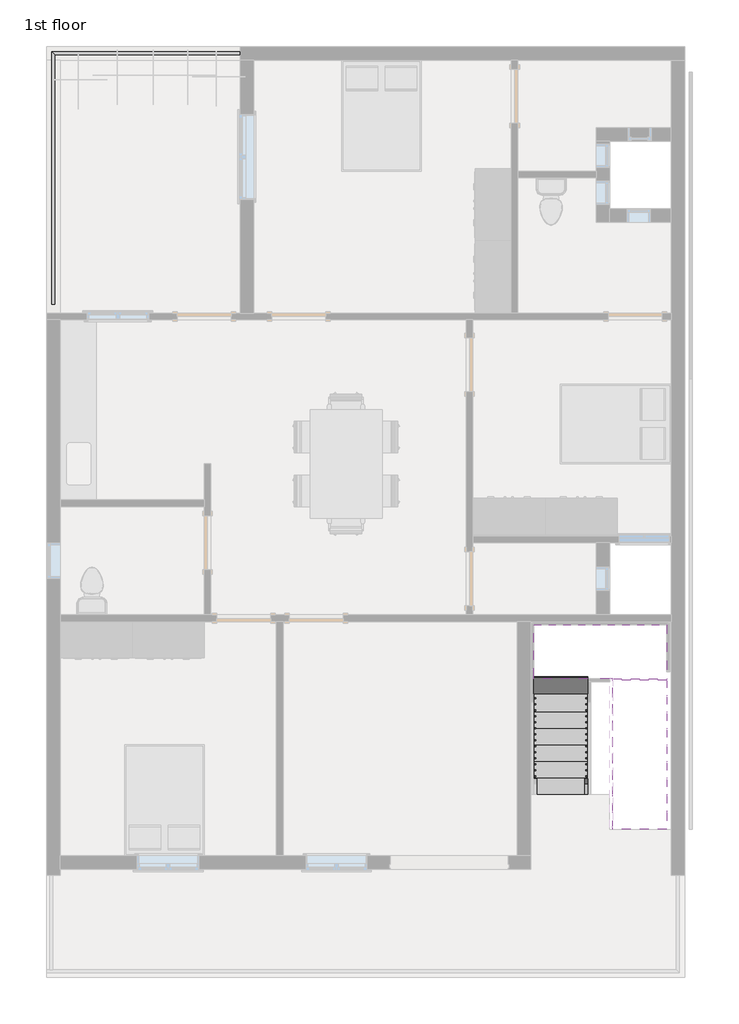
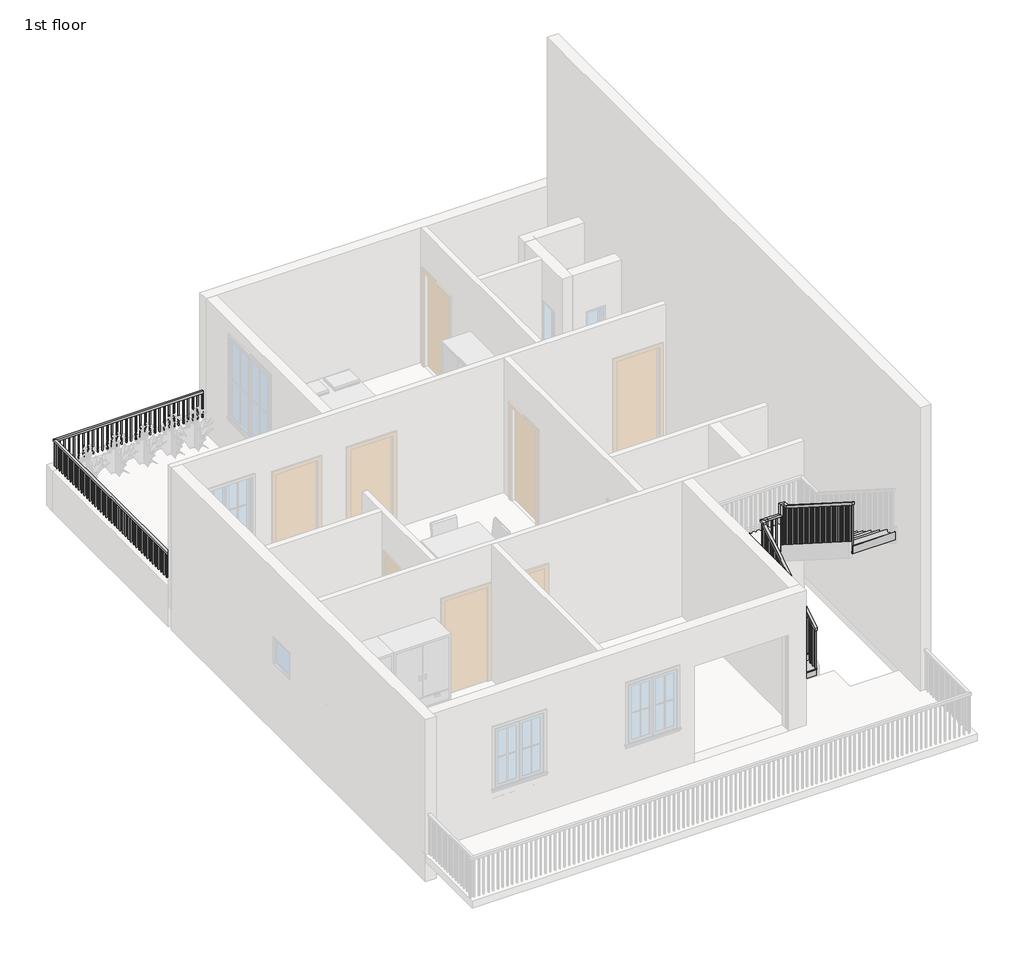
# One storey, part 3 of 5: 2 railings, 2 stair flights, 1 slab.
"""IFC4 building model written with IfcOpenShell, lengths in millimetres."""

from ifc_helpers import new_model, si_unit, frame, origin, place, context, project, spatial, polyline, outline, extrude, faceted_brep, transform, mapped, element, save
from components import non_monolithic_landing_85b13ac5, stair_flight_57d74f5f, stair_flight_b4f684d8

model = new_model("IFC4")

# Units and contexts
model_context = context("Model", 3, world=origin())
ifc_project = project(units=[si_unit("LENGTHUNIT", "METRE", prefix="MILLI")], contexts=[model_context])

# Site, building, storey
site = spatial("IfcSite", under=ifc_project)
building = spatial("IfcBuilding", under=site)
storey = spatial("IfcBuildingStorey", under=building, Name="1st floor", Elevation=3810.0)

# Railings
placement = place(None, origin())
element("IfcRailing", 1, ObjectType="Handrail - Rectangular", at=placement, inside=storey, context=model_context, shape_type="SolidModel", body=[
    faceted_brep([(995.5501403, 157.6257925, 4902.2), (995.5501403, 157.6257925, 4841.986276), (1046.3501403, 157.6257925, 4841.986276), (1046.3501403, 157.6257925, 4902.2), (995.5501403, 2037.2257925, 6098.3090909), (995.5501403, 2088.0257925, 6070.4226396), (1046.3501403, 2088.0257925, 6070.4226396), (1046.3501403, 2037.2257925, 6098.3090909), (995.5501403, 2037.2257925, 6146.8), (995.5501403, 2088.0257925, 6096.0), (1046.3501403, 2088.0257925, 6096.0), (1046.3501403, 2037.2257925, 6146.8), (995.5501403, 2164.2257925, 6146.8), (995.5501403, 2164.2257925, 6096.0), (1046.3501403, 2113.4257925, 6096.0), (1046.3501403, 2113.4257925, 6146.8), (1122.5501403, 2164.2257925, 6146.8), (1122.5501403, 2164.2257925, 6096.0), (1122.5501403, 2113.4257925, 6096.0), (1122.5501403, 2113.4257925, 6146.8), (1389.2501403, 2164.2257925, 6146.8), (1440.0501403, 2164.2257925, 6096.0), (1440.0501403, 2113.4257925, 6096.0), (1389.2501403, 2113.4257925, 6146.8), (1389.2501403, 2164.2257925, 6373.0909091), (1440.0501403, 2164.2257925, 6322.2909091), (1440.0501403, 2113.4257925, 6322.2909091), (1389.2501403, 2113.4257925, 6373.0909091), (1516.2501403, 2164.2257925, 6373.0909091), (1516.2501403, 2164.2257925, 6322.2909091), (1465.4501403, 2113.4257925, 6322.2909091), (1465.4501403, 2113.4257925, 6373.0909091), (1516.2501403, 2037.2257925, 6373.0909091), (1516.2501403, 2022.4327976, 6322.2909091), (1465.4501403, 2022.4327976, 6322.2909091), (1465.4501403, 2037.2257925, 6373.0909091), (1516.2501403, -401.1742075, 7924.8), (1465.4501403, -401.1742075, 7924.8), (1465.4501403, -401.1742075, 7864.586276), (1516.2501403, -401.1742075, 7864.586276)], [[[0, 1, 2, 3]], [[1, 0, 4, 5]], [[2, 1, 5, 6]], [[3, 2, 6, 7]], [[0, 3, 7, 4]], [[5, 4, 8, 9]], [[6, 5, 9, 10]], [[7, 6, 10, 11]], [[4, 7, 11, 8]], [[9, 8, 12, 13]], [[10, 9, 13, 14]], [[11, 10, 14, 15]], [[8, 11, 15, 12]], [[13, 12, 16, 17]], [[14, 13, 17, 18]], [[15, 14, 18, 19]], [[12, 15, 19, 16]], [[17, 16, 20, 21]], [[18, 17, 21, 22]], [[19, 18, 22, 23]], [[16, 19, 23, 20]], [[21, 20, 24, 25]], [[22, 21, 25, 26]], [[23, 22, 26, 27]], [[20, 23, 27, 24]], [[25, 24, 28, 29]], [[26, 25, 29, 30]], [[27, 26, 30, 31]], [[24, 27, 31, 28]], [[29, 28, 32, 33]], [[30, 29, 33, 34]], [[31, 30, 34, 35]], [[28, 31, 35, 32]], [[36, 37, 38, 39]], [[33, 32, 36, 39]], [[34, 33, 39, 38]], [[35, 34, 38, 37]], [[32, 35, 37, 36]]]),
    extrude(outline(polyline([(-309.0992075, 7805.9930941), (-290.0492075, 7793.8703669), (-290.0492075, 6832.6), (-309.0992075, 6832.6), (-309.0992075, 7805.9930941)])), frame((1481.3251403, 0.0, 0.0), z_axis=(1.0, 0.0, 0.0), x_axis=(0.0, 1.0, 0.0)), (0.0, 0.0, 1.0), 19.05),
    extrude(outline(polyline([(-207.4992075, 7741.3385487), (-188.4492075, 7729.2158214), (-188.4492075, 6832.6), (-207.4992075, 6832.6), (-207.4992075, 7741.3385487)])), frame((1481.3251403, 0.0, 0.0), z_axis=(1.0, 0.0, 0.0), x_axis=(0.0, 1.0, 0.0)), (0.0, 0.0, 1.0), 19.05),
    extrude(outline(polyline([(-105.8992075, 7676.6840032), (-86.8492075, 7664.561276), (-86.8492075, 6654.8), (-105.8992075, 6654.8), (-105.8992075, 7676.6840032)])), frame((1481.3251403, 0.0, 0.0), z_axis=(1.0, 0.0, 0.0), x_axis=(0.0, 1.0, 0.0)), (0.0, 0.0, 1.0), 19.05),
    extrude(outline(polyline([(-4.2992075, 7612.0294578), (14.7507925, 7599.9067305), (14.7507925, 6654.8), (-4.2992075, 6654.8), (-4.2992075, 7612.0294578)])), frame((1481.3251403, 0.0, 0.0), z_axis=(1.0, 0.0, 0.0), x_axis=(0.0, 1.0, 0.0)), (0.0, 0.0, 1.0), 19.05),
    extrude(outline(polyline([(97.3007925, 7547.3749123), (116.3507925, 7535.2521851), (116.3507925, 6654.8), (97.3007925, 6654.8), (97.3007925, 7547.3749123)])), frame((1481.3251403, 0.0, 0.0), z_axis=(1.0, 0.0, 0.0), x_axis=(0.0, 1.0, 0.0)), (0.0, 0.0, 1.0), 19.05),
    extrude(outline(polyline([(198.9007925, 7482.7203669), (217.9507925, 7470.5976396), (217.9507925, 6477.0), (198.9007925, 6477.0), (198.9007925, 7482.7203669)])), frame((1481.3251403, 0.0, 0.0), z_axis=(1.0, 0.0, 0.0), x_axis=(0.0, 1.0, 0.0)), (0.0, 0.0, 1.0), 19.05),
    extrude(outline(polyline([(300.5007925, 7418.0658214), (319.5507925, 7405.9430941), (319.5507925, 6477.0), (300.5007925, 6477.0), (300.5007925, 7418.0658214)])), frame((1481.3251403, 0.0, 0.0), z_axis=(1.0, 0.0, 0.0), x_axis=(0.0, 1.0, 0.0)), (0.0, 0.0, 1.0), 19.05),
    extrude(outline(polyline([(402.1007925, 7353.411276), (421.1507925, 7341.2885487), (421.1507925, 6477.0), (402.1007925, 6477.0), (402.1007925, 7353.411276)])), frame((1481.3251403, 0.0, 0.0), z_axis=(1.0, 0.0, 0.0), x_axis=(0.0, 1.0, 0.0)), (0.0, 0.0, 1.0), 19.05),
    extrude(outline(polyline([(503.7007925, 7288.7567305), (522.7507925, 7276.6340032), (522.7507925, 6299.2), (503.7007925, 6299.2), (503.7007925, 7288.7567305)])), frame((1481.3251403, 0.0, 0.0), z_axis=(1.0, 0.0, 0.0), x_axis=(0.0, 1.0, 0.0)), (0.0, 0.0, 1.0), 19.05),
    extrude(outline(polyline([(605.3007925, 7224.1021851), (624.3507925, 7211.9794578), (624.3507925, 6299.2), (605.3007925, 6299.2), (605.3007925, 7224.1021851)])), frame((1481.3251403, 0.0, 0.0), z_axis=(1.0, 0.0, 0.0), x_axis=(0.0, 1.0, 0.0)), (0.0, 0.0, 1.0), 19.05),
    extrude(outline(polyline([(706.9007925, 7159.4476396), (725.9507925, 7147.3249123), (725.9507925, 6299.2), (706.9007925, 6299.2), (706.9007925, 7159.4476396)])), frame((1481.3251403, 0.0, 0.0), z_axis=(1.0, 0.0, 0.0), x_axis=(0.0, 1.0, 0.0)), (0.0, 0.0, 1.0), 19.05),
    extrude(outline(polyline([(808.5007925, 7094.7930941), (827.5507925, 7082.6703669), (827.5507925, 6121.4), (808.5007925, 6121.4), (808.5007925, 7094.7930941)])), frame((1481.3251403, 0.0, 0.0), z_axis=(1.0, 0.0, 0.0), x_axis=(0.0, 1.0, 0.0)), (0.0, 0.0, 1.0), 19.05),
    extrude(outline(polyline([(910.1007925, 7030.1385487), (929.1507925, 7018.0158214), (929.1507925, 6121.4), (910.1007925, 6121.4), (910.1007925, 7030.1385487)])), frame((1481.3251403, 0.0, 0.0), z_axis=(1.0, 0.0, 0.0), x_axis=(0.0, 1.0, 0.0)), (0.0, 0.0, 1.0), 19.05),
    extrude(outline(polyline([(1011.7007925, 6965.4840032), (1030.7507925, 6953.361276), (1030.7507925, 5943.6), (1011.7007925, 5943.6), (1011.7007925, 6965.4840032)])), frame((1481.3251403, 0.0, 0.0), z_axis=(1.0, 0.0, 0.0), x_axis=(0.0, 1.0, 0.0)), (0.0, 0.0, 1.0), 19.05),
    extrude(outline(polyline([(1113.3007925, 6900.8294578), (1132.3507925, 6888.7067305), (1132.3507925, 5943.6), (1113.3007925, 5943.6), (1113.3007925, 6900.8294578)])), frame((1481.3251403, 0.0, 0.0), z_axis=(1.0, 0.0, 0.0), x_axis=(0.0, 1.0, 0.0)), (0.0, 0.0, 1.0), 19.05),
    extrude(outline(polyline([(1214.9007925, 6836.1749123), (1233.9507925, 6824.0521851), (1233.9507925, 5943.6), (1214.9007925, 5943.6), (1214.9007925, 6836.1749123)])), frame((1481.3251403, 0.0, 0.0), z_axis=(1.0, 0.0, 0.0), x_axis=(0.0, 1.0, 0.0)), (0.0, 0.0, 1.0), 19.05),
    extrude(outline(polyline([(1316.5007925, 6771.5203669), (1335.5507925, 6759.3976396), (1335.5507925, 5765.8), (1316.5007925, 5765.8), (1316.5007925, 6771.5203669)])), frame((1481.3251403, 0.0, 0.0), z_axis=(1.0, 0.0, 0.0), x_axis=(0.0, 1.0, 0.0)), (0.0, 0.0, 1.0), 19.05),
    extrude(outline(polyline([(1418.1007925, 6706.8658214), (1437.1507925, 6694.7430941), (1437.1507925, 5765.8), (1418.1007925, 5765.8), (1418.1007925, 6706.8658214)])), frame((1481.3251403, 0.0, 0.0), z_axis=(1.0, 0.0, 0.0), x_axis=(0.0, 1.0, 0.0)), (0.0, 0.0, 1.0), 19.05),
    extrude(outline(polyline([(1519.7007925, 6642.211276), (1538.7507925, 6630.0885487), (1538.7507925, 5765.8), (1519.7007925, 5765.8), (1519.7007925, 6642.211276)])), frame((1481.3251403, 0.0, 0.0), z_axis=(1.0, 0.0, 0.0), x_axis=(0.0, 1.0, 0.0)), (0.0, 0.0, 1.0), 19.05),
    extrude(outline(polyline([(1621.3007925, 6577.5567305), (1640.3507925, 6565.4340032), (1640.3507925, 5588.0), (1621.3007925, 5588.0), (1621.3007925, 6577.5567305)])), frame((1481.3251403, 0.0, 0.0), z_axis=(1.0, 0.0, 0.0), x_axis=(0.0, 1.0, 0.0)), (0.0, 0.0, 1.0), 19.05),
    extrude(outline(polyline([(1722.9007925, 6512.9021851), (1741.9507925, 6500.7794578), (1741.9507925, 5588.0), (1722.9007925, 5588.0), (1722.9007925, 6512.9021851)])), frame((1481.3251403, 0.0, 0.0), z_axis=(1.0, 0.0, 0.0), x_axis=(0.0, 1.0, 0.0)), (0.0, 0.0, 1.0), 19.05),
    extrude(outline(polyline([(1824.5007925, 6448.2476396), (1843.5507925, 6436.1249123), (1843.5507925, 5588.0), (1824.5007925, 5588.0), (1824.5007925, 6448.2476396)])), frame((1481.3251403, 0.0, 0.0), z_axis=(1.0, 0.0, 0.0), x_axis=(0.0, 1.0, 0.0)), (0.0, 0.0, 1.0), 19.05),
    extrude(outline(polyline([(1926.1007925, 6383.5930941), (1945.1507925, 6371.4703669), (1945.1507925, 5410.2), (1926.1007925, 5410.2), (1926.1007925, 6383.5930941)])), frame((1481.3251403, 0.0, 0.0), z_axis=(1.0, 0.0, 0.0), x_axis=(0.0, 1.0, 0.0)), (0.0, 0.0, 1.0), 19.05),
    extrude(outline(polyline([(2027.7007925, 6318.9385487), (2046.7507925, 6306.8158214), (2046.7507925, 5410.2), (2027.7007925, 5410.2), (2027.7007925, 6318.9385487)])), frame((1481.3251403, 0.0, 0.0), z_axis=(1.0, 0.0, 0.0), x_axis=(0.0, 1.0, 0.0)), (0.0, 0.0, 1.0), 19.05),
    extrude(outline(polyline([(1417.8251403, 2129.3007925), (1417.8251403, 2148.3507925), (1436.8751403, 2148.3507925), (1436.8751403, 2129.3007925), (1417.8251403, 2129.3007925)])), frame((0.0, 0.0, 5232.4), z_axis=(0.0, 0.0, 1.0), x_axis=(1.0, 0.0, 0.0)), (0.0, 0.0, 1.0), 1089.8909091),
    extrude(outline(polyline([(1316.2251403, 2129.3007925), (1316.2251403, 2148.3507925), (1335.2751403, 2148.3507925), (1335.2751403, 2129.3007925), (1316.2251403, 2129.3007925)])), frame((0.0, 0.0, 5232.4), z_axis=(0.0, 0.0, 1.0), x_axis=(1.0, 0.0, 0.0)), (0.0, 0.0, 1.0), 863.6),
    extrude(outline(polyline([(1214.6251403, 2129.3007925), (1214.6251403, 2148.3507925), (1233.6751403, 2148.3507925), (1233.6751403, 2129.3007925), (1214.6251403, 2129.3007925)])), frame((0.0, 0.0, 5232.4), z_axis=(0.0, 0.0, 1.0), x_axis=(1.0, 0.0, 0.0)), (0.0, 0.0, 1.0), 863.6),
    extrude(outline(polyline([(1113.0251403, 2129.3007925), (1113.0251403, 2148.3507925), (1132.0751403, 2148.3507925), (1132.0751403, 2129.3007925), (1113.0251403, 2129.3007925)])), frame((0.0, 0.0, 5232.4), z_axis=(0.0, 0.0, 1.0), x_axis=(1.0, 0.0, 0.0)), (0.0, 0.0, 1.0), 863.6),
    extrude(outline(polyline([(1030.4751403, 2078.5007925), (1011.4251403, 2078.5007925), (1011.4251403, 2097.5507925), (1030.4751403, 2097.5507925), (1030.4751403, 2078.5007925)])), frame((0.0, 0.0, 5054.6), z_axis=(0.0, 0.0, 1.0), x_axis=(1.0, 0.0, 0.0)), (0.0, 0.0, 1.0), 1041.4),
    extrude(outline(polyline([(1976.9007925, 5999.7067305), (1995.9507925, 6011.8294578), (1995.9507925, 5054.6), (1976.9007925, 5054.6), (1976.9007925, 5999.7067305)])), frame((1011.4251403, 0.0, 0.0), z_axis=(1.0, 0.0, 0.0), x_axis=(0.0, 1.0, 0.0)), (0.0, 0.0, 1.0), 19.05),
    extrude(outline(polyline([(1875.3007925, 5935.0521851), (1894.3507925, 5947.1749123), (1894.3507925, 5054.6), (1875.3007925, 5054.6), (1875.3007925, 5935.0521851)])), frame((1011.4251403, 0.0, 0.0), z_axis=(1.0, 0.0, 0.0), x_axis=(0.0, 1.0, 0.0)), (0.0, 0.0, 1.0), 19.05),
    extrude(outline(polyline([(1773.7007925, 5870.3976396), (1792.7507925, 5882.5203669), (1792.7507925, 4876.8), (1773.7007925, 4876.8), (1773.7007925, 5870.3976396)])), frame((1011.4251403, 0.0, 0.0), z_axis=(1.0, 0.0, 0.0), x_axis=(0.0, 1.0, 0.0)), (0.0, 0.0, 1.0), 19.05),
    extrude(outline(polyline([(1672.1007925, 5805.7430941), (1691.1507925, 5817.8658214), (1691.1507925, 4876.8), (1672.1007925, 4876.8), (1672.1007925, 5805.7430941)])), frame((1011.4251403, 0.0, 0.0), z_axis=(1.0, 0.0, 0.0), x_axis=(0.0, 1.0, 0.0)), (0.0, 0.0, 1.0), 19.05),
    extrude(outline(polyline([(1570.5007925, 5741.0885487), (1589.5507925, 5753.211276), (1589.5507925, 4876.8), (1570.5007925, 4876.8), (1570.5007925, 5741.0885487)])), frame((1011.4251403, 0.0, 0.0), z_axis=(1.0, 0.0, 0.0), x_axis=(0.0, 1.0, 0.0)), (0.0, 0.0, 1.0), 19.05),
    extrude(outline(polyline([(1468.9007925, 5676.4340032), (1487.9507925, 5688.5567305), (1487.9507925, 4699.0), (1468.9007925, 4699.0), (1468.9007925, 5676.4340032)])), frame((1011.4251403, 0.0, 0.0), z_axis=(1.0, 0.0, 0.0), x_axis=(0.0, 1.0, 0.0)), (0.0, 0.0, 1.0), 19.05),
    extrude(outline(polyline([(1367.3007925, 5611.7794578), (1386.3507925, 5623.9021851), (1386.3507925, 4699.0), (1367.3007925, 4699.0), (1367.3007925, 5611.7794578)])), frame((1011.4251403, 0.0, 0.0), z_axis=(1.0, 0.0, 0.0), x_axis=(0.0, 1.0, 0.0)), (0.0, 0.0, 1.0), 19.05),
    extrude(outline(polyline([(1265.7007925, 5547.1249123), (1284.7507925, 5559.2476396), (1284.7507925, 4699.0), (1265.7007925, 4699.0), (1265.7007925, 5547.1249123)])), frame((1011.4251403, 0.0, 0.0), z_axis=(1.0, 0.0, 0.0), x_axis=(0.0, 1.0, 0.0)), (0.0, 0.0, 1.0), 19.05),
    extrude(outline(polyline([(1164.1007925, 5482.4703669), (1183.1507925, 5494.5930941), (1183.1507925, 4521.2), (1164.1007925, 4521.2), (1164.1007925, 5482.4703669)])), frame((1011.4251403, 0.0, 0.0), z_axis=(1.0, 0.0, 0.0), x_axis=(0.0, 1.0, 0.0)), (0.0, 0.0, 1.0), 19.05),
    extrude(outline(polyline([(1062.5007925, 5417.8158214), (1081.5507925, 5429.9385487), (1081.5507925, 4521.2), (1062.5007925, 4521.2), (1062.5007925, 5417.8158214)])), frame((1011.4251403, 0.0, 0.0), z_axis=(1.0, 0.0, 0.0), x_axis=(0.0, 1.0, 0.0)), (0.0, 0.0, 1.0), 19.05),
    extrude(outline(polyline([(960.9007925, 5353.161276), (979.9507925, 5365.2840032), (979.9507925, 4343.4), (960.9007925, 4343.4), (960.9007925, 5353.161276)])), frame((1011.4251403, 0.0, 0.0), z_axis=(1.0, 0.0, 0.0), x_axis=(0.0, 1.0, 0.0)), (0.0, 0.0, 1.0), 19.05),
    extrude(outline(polyline([(859.3007925, 5288.5067305), (878.3507925, 5300.6294578), (878.3507925, 4343.4), (859.3007925, 4343.4), (859.3007925, 5288.5067305)])), frame((1011.4251403, 0.0, 0.0), z_axis=(1.0, 0.0, 0.0), x_axis=(0.0, 1.0, 0.0)), (0.0, 0.0, 1.0), 19.05),
    extrude(outline(polyline([(757.7007925, 5223.8521851), (776.7507925, 5235.9749123), (776.7507925, 4343.4), (757.7007925, 4343.4), (757.7007925, 5223.8521851)])), frame((1011.4251403, 0.0, 0.0), z_axis=(1.0, 0.0, 0.0), x_axis=(0.0, 1.0, 0.0)), (0.0, 0.0, 1.0), 19.05),
    extrude(outline(polyline([(656.1007925, 5159.1976396), (675.1507925, 5171.3203669), (675.1507925, 4165.6), (656.1007925, 4165.6), (656.1007925, 5159.1976396)])), frame((1011.4251403, 0.0, 0.0), z_axis=(1.0, 0.0, 0.0), x_axis=(0.0, 1.0, 0.0)), (0.0, 0.0, 1.0), 19.05),
    extrude(outline(polyline([(554.5007925, 5094.5430941), (573.5507925, 5106.6658214), (573.5507925, 4165.6), (554.5007925, 4165.6), (554.5007925, 5094.5430941)])), frame((1011.4251403, 0.0, 0.0), z_axis=(1.0, 0.0, 0.0), x_axis=(0.0, 1.0, 0.0)), (0.0, 0.0, 1.0), 19.05),
    extrude(outline(polyline([(452.9007925, 5029.8885487), (471.9507925, 5042.011276), (471.9507925, 4165.6), (452.9007925, 4165.6), (452.9007925, 5029.8885487)])), frame((1011.4251403, 0.0, 0.0), z_axis=(1.0, 0.0, 0.0), x_axis=(0.0, 1.0, 0.0)), (0.0, 0.0, 1.0), 19.05),
    extrude(outline(polyline([(351.3007925, 4965.2340032), (370.3507925, 4977.3567305), (370.3507925, 3987.8), (351.3007925, 3987.8), (351.3007925, 4965.2340032)])), frame((1011.4251403, 0.0, 0.0), z_axis=(1.0, 0.0, 0.0), x_axis=(0.0, 1.0, 0.0)), (0.0, 0.0, 1.0), 19.05),
    extrude(outline(polyline([(249.7007925, 4900.5794578), (268.7507925, 4912.7021851), (268.7507925, 3987.8), (249.7007925, 3987.8), (249.7007925, 4900.5794578)])), frame((1011.4251403, 0.0, 0.0), z_axis=(1.0, 0.0, 0.0), x_axis=(0.0, 1.0, 0.0)), (0.0, 0.0, 1.0), 19.05),
    extrude(outline(polyline([(1481.3251403, 2129.3007925), (1481.3251403, 2148.3507925), (1500.3751403, 2148.3507925), (1500.3751403, 2129.3007925), (1481.3251403, 2129.3007925)])), frame((0.0, 0.0, 5232.4), z_axis=(0.0, 0.0, 1.0), x_axis=(1.0, 0.0, 0.0)), (0.0, 0.0, 1.0), 1089.8909091),
    extrude(outline(polyline([(1030.4751403, 2129.3007925), (1011.4251403, 2129.3007925), (1011.4251403, 2148.3507925), (1030.4751403, 2148.3507925), (1030.4751403, 2129.3007925)])), frame((0.0, 0.0, 5232.4), z_axis=(0.0, 0.0, 1.0), x_axis=(1.0, 0.0, 0.0)), (0.0, 0.0, 1.0), 863.6),
    extrude(outline(polyline([(-401.1742075, 7864.586276), (-382.1242075, 7852.4635487), (-382.1242075, 6832.6), (-401.1742075, 6832.6), (-401.1742075, 7864.586276)])), frame((1481.3251403, 0.0, 0.0), z_axis=(1.0, 0.0, 0.0), x_axis=(0.0, 1.0, 0.0)), (0.0, 0.0, 1.0), 19.05),
    extrude(outline(polyline([(157.6257925, 4841.986276), (176.6757925, 4854.1090032), (176.6757925, 3987.8), (157.6257925, 3987.8), (157.6257925, 4841.986276)])), frame((1011.4251403, 0.0, 0.0), z_axis=(1.0, 0.0, 0.0), x_axis=(0.0, 1.0, 0.0)), (0.0, 0.0, 1.0), 19.05),
])
element("IfcRailing", 2, ObjectType="Handrail - Rectangular", at=placement, inside=storey, context=model_context, shape_type="SolidModel", body=[
    faceted_brep([(-8021.4498597, 8450.7257925, 4724.4), (-8021.4498597, 8450.7257925, 4673.6), (-7970.6498597, 8450.7257925, 4673.6), (-7970.6498597, 8450.7257925, 4724.4), (-8021.4498597, 12717.9257925, 4724.4), (-8021.4498597, 12717.9257925, 4673.6), (-7970.6498597, 12667.1257925, 4673.6), (-7970.6498597, 12667.1257925, 4724.4), (-4795.6498597, 12717.9257925, 4724.4), (-4795.6498597, 12667.1257925, 4724.4), (-4795.6498597, 12667.1257925, 4673.6), (-4795.6498597, 12717.9257925, 4673.6)], [[[0, 1, 2, 3]], [[1, 0, 4, 5]], [[2, 1, 5, 6]], [[3, 2, 6, 7]], [[0, 3, 7, 4]], [[8, 9, 10, 11]], [[5, 4, 8, 11]], [[6, 5, 11, 10]], [[7, 6, 10, 9]], [[4, 7, 9, 8]]]),
    extrude(outline(polyline([(-4855.9748597, 12683.0007925), (-4855.9748597, 12702.0507925), (-4836.9248597, 12702.0507925), (-4836.9248597, 12683.0007925), (-4855.9748597, 12683.0007925)])), frame((0.0, 0.0, 3810.0), z_axis=(0.0, 0.0, 1.0), x_axis=(1.0, 0.0, 0.0)), (0.0, 0.0, 1.0), 863.6),
    extrude(outline(polyline([(-4957.5748597, 12683.0007925), (-4957.5748597, 12702.0507925), (-4938.5248597, 12702.0507925), (-4938.5248597, 12683.0007925), (-4957.5748597, 12683.0007925)])), frame((0.0, 0.0, 3810.0), z_axis=(0.0, 0.0, 1.0), x_axis=(1.0, 0.0, 0.0)), (0.0, 0.0, 1.0), 863.6),
    extrude(outline(polyline([(-5059.1748597, 12683.0007925), (-5059.1748597, 12702.0507925), (-5040.1248597, 12702.0507925), (-5040.1248597, 12683.0007925), (-5059.1748597, 12683.0007925)])), frame((0.0, 0.0, 3810.0), z_axis=(0.0, 0.0, 1.0), x_axis=(1.0, 0.0, 0.0)), (0.0, 0.0, 1.0), 863.6),
    extrude(outline(polyline([(-5160.7748597, 12683.0007925), (-5160.7748597, 12702.0507925), (-5141.7248597, 12702.0507925), (-5141.7248597, 12683.0007925), (-5160.7748597, 12683.0007925)])), frame((0.0, 0.0, 3810.0), z_axis=(0.0, 0.0, 1.0), x_axis=(1.0, 0.0, 0.0)), (0.0, 0.0, 1.0), 863.6),
    extrude(outline(polyline([(-5262.3748597, 12683.0007925), (-5262.3748597, 12702.0507925), (-5243.3248597, 12702.0507925), (-5243.3248597, 12683.0007925), (-5262.3748597, 12683.0007925)])), frame((0.0, 0.0, 3810.0), z_axis=(0.0, 0.0, 1.0), x_axis=(1.0, 0.0, 0.0)), (0.0, 0.0, 1.0), 863.6),
    extrude(outline(polyline([(-5363.9748597, 12683.0007925), (-5363.9748597, 12702.0507925), (-5344.9248597, 12702.0507925), (-5344.9248597, 12683.0007925), (-5363.9748597, 12683.0007925)])), frame((0.0, 0.0, 3810.0), z_axis=(0.0, 0.0, 1.0), x_axis=(1.0, 0.0, 0.0)), (0.0, 0.0, 1.0), 863.6),
    extrude(outline(polyline([(-5465.5748597, 12683.0007925), (-5465.5748597, 12702.0507925), (-5446.5248597, 12702.0507925), (-5446.5248597, 12683.0007925), (-5465.5748597, 12683.0007925)])), frame((0.0, 0.0, 3810.0), z_axis=(0.0, 0.0, 1.0), x_axis=(1.0, 0.0, 0.0)), (0.0, 0.0, 1.0), 863.6),
    extrude(outline(polyline([(-5567.1748597, 12683.0007925), (-5567.1748597, 12702.0507925), (-5548.1248597, 12702.0507925), (-5548.1248597, 12683.0007925), (-5567.1748597, 12683.0007925)])), frame((0.0, 0.0, 3810.0), z_axis=(0.0, 0.0, 1.0), x_axis=(1.0, 0.0, 0.0)), (0.0, 0.0, 1.0), 863.6),
    extrude(outline(polyline([(-5668.7748597, 12683.0007925), (-5668.7748597, 12702.0507925), (-5649.7248597, 12702.0507925), (-5649.7248597, 12683.0007925), (-5668.7748597, 12683.0007925)])), frame((0.0, 0.0, 3810.0), z_axis=(0.0, 0.0, 1.0), x_axis=(1.0, 0.0, 0.0)), (0.0, 0.0, 1.0), 863.6),
    extrude(outline(polyline([(-5770.3748597, 12683.0007925), (-5770.3748597, 12702.0507925), (-5751.3248597, 12702.0507925), (-5751.3248597, 12683.0007925), (-5770.3748597, 12683.0007925)])), frame((0.0, 0.0, 3810.0), z_axis=(0.0, 0.0, 1.0), x_axis=(1.0, 0.0, 0.0)), (0.0, 0.0, 1.0), 863.6),
    extrude(outline(polyline([(-5871.9748597, 12683.0007925), (-5871.9748597, 12702.0507925), (-5852.9248597, 12702.0507925), (-5852.9248597, 12683.0007925), (-5871.9748597, 12683.0007925)])), frame((0.0, 0.0, 3810.0), z_axis=(0.0, 0.0, 1.0), x_axis=(1.0, 0.0, 0.0)), (0.0, 0.0, 1.0), 863.6),
    extrude(outline(polyline([(-5973.5748597, 12683.0007925), (-5973.5748597, 12702.0507925), (-5954.5248597, 12702.0507925), (-5954.5248597, 12683.0007925), (-5973.5748597, 12683.0007925)])), frame((0.0, 0.0, 3810.0), z_axis=(0.0, 0.0, 1.0), x_axis=(1.0, 0.0, 0.0)), (0.0, 0.0, 1.0), 863.6),
    extrude(outline(polyline([(-6075.1748597, 12683.0007925), (-6075.1748597, 12702.0507925), (-6056.1248597, 12702.0507925), (-6056.1248597, 12683.0007925), (-6075.1748597, 12683.0007925)])), frame((0.0, 0.0, 3810.0), z_axis=(0.0, 0.0, 1.0), x_axis=(1.0, 0.0, 0.0)), (0.0, 0.0, 1.0), 863.6),
    extrude(outline(polyline([(-6176.7748597, 12683.0007925), (-6176.7748597, 12702.0507925), (-6157.7248597, 12702.0507925), (-6157.7248597, 12683.0007925), (-6176.7748597, 12683.0007925)])), frame((0.0, 0.0, 3810.0), z_axis=(0.0, 0.0, 1.0), x_axis=(1.0, 0.0, 0.0)), (0.0, 0.0, 1.0), 863.6),
    extrude(outline(polyline([(-6278.3748597, 12683.0007925), (-6278.3748597, 12702.0507925), (-6259.3248597, 12702.0507925), (-6259.3248597, 12683.0007925), (-6278.3748597, 12683.0007925)])), frame((0.0, 0.0, 3810.0), z_axis=(0.0, 0.0, 1.0), x_axis=(1.0, 0.0, 0.0)), (0.0, 0.0, 1.0), 863.6),
    extrude(outline(polyline([(-6379.9748597, 12683.0007925), (-6379.9748597, 12702.0507925), (-6360.9248597, 12702.0507925), (-6360.9248597, 12683.0007925), (-6379.9748597, 12683.0007925)])), frame((0.0, 0.0, 3810.0), z_axis=(0.0, 0.0, 1.0), x_axis=(1.0, 0.0, 0.0)), (0.0, 0.0, 1.0), 863.6),
    extrude(outline(polyline([(-6481.5748597, 12683.0007925), (-6481.5748597, 12702.0507925), (-6462.5248597, 12702.0507925), (-6462.5248597, 12683.0007925), (-6481.5748597, 12683.0007925)])), frame((0.0, 0.0, 3810.0), z_axis=(0.0, 0.0, 1.0), x_axis=(1.0, 0.0, 0.0)), (0.0, 0.0, 1.0), 863.6),
    extrude(outline(polyline([(-6583.1748597, 12683.0007925), (-6583.1748597, 12702.0507925), (-6564.1248597, 12702.0507925), (-6564.1248597, 12683.0007925), (-6583.1748597, 12683.0007925)])), frame((0.0, 0.0, 3810.0), z_axis=(0.0, 0.0, 1.0), x_axis=(1.0, 0.0, 0.0)), (0.0, 0.0, 1.0), 863.6),
    extrude(outline(polyline([(-6684.7748597, 12683.0007925), (-6684.7748597, 12702.0507925), (-6665.7248597, 12702.0507925), (-6665.7248597, 12683.0007925), (-6684.7748597, 12683.0007925)])), frame((0.0, 0.0, 3810.0), z_axis=(0.0, 0.0, 1.0), x_axis=(1.0, 0.0, 0.0)), (0.0, 0.0, 1.0), 863.6),
    extrude(outline(polyline([(-6786.3748597, 12683.0007925), (-6786.3748597, 12702.0507925), (-6767.3248597, 12702.0507925), (-6767.3248597, 12683.0007925), (-6786.3748597, 12683.0007925)])), frame((0.0, 0.0, 3810.0), z_axis=(0.0, 0.0, 1.0), x_axis=(1.0, 0.0, 0.0)), (0.0, 0.0, 1.0), 863.6),
    extrude(outline(polyline([(-6887.9748597, 12683.0007925), (-6887.9748597, 12702.0507925), (-6868.9248597, 12702.0507925), (-6868.9248597, 12683.0007925), (-6887.9748597, 12683.0007925)])), frame((0.0, 0.0, 3810.0), z_axis=(0.0, 0.0, 1.0), x_axis=(1.0, 0.0, 0.0)), (0.0, 0.0, 1.0), 863.6),
    extrude(outline(polyline([(-6989.5748597, 12683.0007925), (-6989.5748597, 12702.0507925), (-6970.5248597, 12702.0507925), (-6970.5248597, 12683.0007925), (-6989.5748597, 12683.0007925)])), frame((0.0, 0.0, 3810.0), z_axis=(0.0, 0.0, 1.0), x_axis=(1.0, 0.0, 0.0)), (0.0, 0.0, 1.0), 863.6),
    extrude(outline(polyline([(-7091.1748597, 12683.0007925), (-7091.1748597, 12702.0507925), (-7072.1248597, 12702.0507925), (-7072.1248597, 12683.0007925), (-7091.1748597, 12683.0007925)])), frame((0.0, 0.0, 3810.0), z_axis=(0.0, 0.0, 1.0), x_axis=(1.0, 0.0, 0.0)), (0.0, 0.0, 1.0), 863.6),
    extrude(outline(polyline([(-7192.7748597, 12683.0007925), (-7192.7748597, 12702.0507925), (-7173.7248597, 12702.0507925), (-7173.7248597, 12683.0007925), (-7192.7748597, 12683.0007925)])), frame((0.0, 0.0, 3810.0), z_axis=(0.0, 0.0, 1.0), x_axis=(1.0, 0.0, 0.0)), (0.0, 0.0, 1.0), 863.6),
    extrude(outline(polyline([(-7294.3748597, 12683.0007925), (-7294.3748597, 12702.0507925), (-7275.3248597, 12702.0507925), (-7275.3248597, 12683.0007925), (-7294.3748597, 12683.0007925)])), frame((0.0, 0.0, 3810.0), z_axis=(0.0, 0.0, 1.0), x_axis=(1.0, 0.0, 0.0)), (0.0, 0.0, 1.0), 863.6),
    extrude(outline(polyline([(-7395.9748597, 12683.0007925), (-7395.9748597, 12702.0507925), (-7376.9248597, 12702.0507925), (-7376.9248597, 12683.0007925), (-7395.9748597, 12683.0007925)])), frame((0.0, 0.0, 3810.0), z_axis=(0.0, 0.0, 1.0), x_axis=(1.0, 0.0, 0.0)), (0.0, 0.0, 1.0), 863.6),
    extrude(outline(polyline([(-7497.5748597, 12683.0007925), (-7497.5748597, 12702.0507925), (-7478.5248597, 12702.0507925), (-7478.5248597, 12683.0007925), (-7497.5748597, 12683.0007925)])), frame((0.0, 0.0, 3810.0), z_axis=(0.0, 0.0, 1.0), x_axis=(1.0, 0.0, 0.0)), (0.0, 0.0, 1.0), 863.6),
    extrude(outline(polyline([(-7599.1748597, 12683.0007925), (-7599.1748597, 12702.0507925), (-7580.1248597, 12702.0507925), (-7580.1248597, 12683.0007925), (-7599.1748597, 12683.0007925)])), frame((0.0, 0.0, 3810.0), z_axis=(0.0, 0.0, 1.0), x_axis=(1.0, 0.0, 0.0)), (0.0, 0.0, 1.0), 863.6),
    extrude(outline(polyline([(-7700.7748597, 12683.0007925), (-7700.7748597, 12702.0507925), (-7681.7248597, 12702.0507925), (-7681.7248597, 12683.0007925), (-7700.7748597, 12683.0007925)])), frame((0.0, 0.0, 3810.0), z_axis=(0.0, 0.0, 1.0), x_axis=(1.0, 0.0, 0.0)), (0.0, 0.0, 1.0), 863.6),
    extrude(outline(polyline([(-7802.3748597, 12683.0007925), (-7802.3748597, 12702.0507925), (-7783.3248597, 12702.0507925), (-7783.3248597, 12683.0007925), (-7802.3748597, 12683.0007925)])), frame((0.0, 0.0, 3810.0), z_axis=(0.0, 0.0, 1.0), x_axis=(1.0, 0.0, 0.0)), (0.0, 0.0, 1.0), 863.6),
    extrude(outline(polyline([(-7903.9748597, 12683.0007925), (-7903.9748597, 12702.0507925), (-7884.9248597, 12702.0507925), (-7884.9248597, 12683.0007925), (-7903.9748597, 12683.0007925)])), frame((0.0, 0.0, 3810.0), z_axis=(0.0, 0.0, 1.0), x_axis=(1.0, 0.0, 0.0)), (0.0, 0.0, 1.0), 863.6),
    extrude(outline(polyline([(-7986.5248597, 12606.8007925), (-8005.5748597, 12606.8007925), (-8005.5748597, 12625.8507925), (-7986.5248597, 12625.8507925), (-7986.5248597, 12606.8007925)])), frame((0.0, 0.0, 3810.0), z_axis=(0.0, 0.0, 1.0), x_axis=(1.0, 0.0, 0.0)), (0.0, 0.0, 1.0), 863.6),
    extrude(outline(polyline([(-7986.5248597, 12505.2007925), (-8005.5748597, 12505.2007925), (-8005.5748597, 12524.2507925), (-7986.5248597, 12524.2507925), (-7986.5248597, 12505.2007925)])), frame((0.0, 0.0, 3810.0), z_axis=(0.0, 0.0, 1.0), x_axis=(1.0, 0.0, 0.0)), (0.0, 0.0, 1.0), 863.6),
    extrude(outline(polyline([(-7986.5248597, 12403.6007925), (-8005.5748597, 12403.6007925), (-8005.5748597, 12422.6507925), (-7986.5248597, 12422.6507925), (-7986.5248597, 12403.6007925)])), frame((0.0, 0.0, 3810.0), z_axis=(0.0, 0.0, 1.0), x_axis=(1.0, 0.0, 0.0)), (0.0, 0.0, 1.0), 863.6),
    extrude(outline(polyline([(-7986.5248597, 12302.0007925), (-8005.5748597, 12302.0007925), (-8005.5748597, 12321.0507925), (-7986.5248597, 12321.0507925), (-7986.5248597, 12302.0007925)])), frame((0.0, 0.0, 3810.0), z_axis=(0.0, 0.0, 1.0), x_axis=(1.0, 0.0, 0.0)), (0.0, 0.0, 1.0), 863.6),
    extrude(outline(polyline([(-7986.5248597, 12200.4007925), (-8005.5748597, 12200.4007925), (-8005.5748597, 12219.4507925), (-7986.5248597, 12219.4507925), (-7986.5248597, 12200.4007925)])), frame((0.0, 0.0, 3810.0), z_axis=(0.0, 0.0, 1.0), x_axis=(1.0, 0.0, 0.0)), (0.0, 0.0, 1.0), 863.6),
    extrude(outline(polyline([(-7986.5248597, 12098.8007925), (-8005.5748597, 12098.8007925), (-8005.5748597, 12117.8507925), (-7986.5248597, 12117.8507925), (-7986.5248597, 12098.8007925)])), frame((0.0, 0.0, 3810.0), z_axis=(0.0, 0.0, 1.0), x_axis=(1.0, 0.0, 0.0)), (0.0, 0.0, 1.0), 863.6),
    extrude(outline(polyline([(-7986.5248597, 11997.2007925), (-8005.5748597, 11997.2007925), (-8005.5748597, 12016.2507925), (-7986.5248597, 12016.2507925), (-7986.5248597, 11997.2007925)])), frame((0.0, 0.0, 3810.0), z_axis=(0.0, 0.0, 1.0), x_axis=(1.0, 0.0, 0.0)), (0.0, 0.0, 1.0), 863.6),
    extrude(outline(polyline([(-7986.5248597, 11895.6007925), (-8005.5748597, 11895.6007925), (-8005.5748597, 11914.6507925), (-7986.5248597, 11914.6507925), (-7986.5248597, 11895.6007925)])), frame((0.0, 0.0, 3810.0), z_axis=(0.0, 0.0, 1.0), x_axis=(1.0, 0.0, 0.0)), (0.0, 0.0, 1.0), 863.6),
    extrude(outline(polyline([(-7986.5248597, 11794.0007925), (-8005.5748597, 11794.0007925), (-8005.5748597, 11813.0507925), (-7986.5248597, 11813.0507925), (-7986.5248597, 11794.0007925)])), frame((0.0, 0.0, 3810.0), z_axis=(0.0, 0.0, 1.0), x_axis=(1.0, 0.0, 0.0)), (0.0, 0.0, 1.0), 863.6),
    extrude(outline(polyline([(-7986.5248597, 11692.4007925), (-8005.5748597, 11692.4007925), (-8005.5748597, 11711.4507925), (-7986.5248597, 11711.4507925), (-7986.5248597, 11692.4007925)])), frame((0.0, 0.0, 3810.0), z_axis=(0.0, 0.0, 1.0), x_axis=(1.0, 0.0, 0.0)), (0.0, 0.0, 1.0), 863.6),
    extrude(outline(polyline([(-7986.5248597, 11590.8007925), (-8005.5748597, 11590.8007925), (-8005.5748597, 11609.8507925), (-7986.5248597, 11609.8507925), (-7986.5248597, 11590.8007925)])), frame((0.0, 0.0, 3810.0), z_axis=(0.0, 0.0, 1.0), x_axis=(1.0, 0.0, 0.0)), (0.0, 0.0, 1.0), 863.6),
    extrude(outline(polyline([(-7986.5248597, 11489.2007925), (-8005.5748597, 11489.2007925), (-8005.5748597, 11508.2507925), (-7986.5248597, 11508.2507925), (-7986.5248597, 11489.2007925)])), frame((0.0, 0.0, 3810.0), z_axis=(0.0, 0.0, 1.0), x_axis=(1.0, 0.0, 0.0)), (0.0, 0.0, 1.0), 863.6),
    extrude(outline(polyline([(-7986.5248597, 11387.6007925), (-8005.5748597, 11387.6007925), (-8005.5748597, 11406.6507925), (-7986.5248597, 11406.6507925), (-7986.5248597, 11387.6007925)])), frame((0.0, 0.0, 3810.0), z_axis=(0.0, 0.0, 1.0), x_axis=(1.0, 0.0, 0.0)), (0.0, 0.0, 1.0), 863.6),
    extrude(outline(polyline([(-7986.5248597, 11286.0007925), (-8005.5748597, 11286.0007925), (-8005.5748597, 11305.0507925), (-7986.5248597, 11305.0507925), (-7986.5248597, 11286.0007925)])), frame((0.0, 0.0, 3810.0), z_axis=(0.0, 0.0, 1.0), x_axis=(1.0, 0.0, 0.0)), (0.0, 0.0, 1.0), 863.6),
    extrude(outline(polyline([(-7986.5248597, 11184.4007925), (-8005.5748597, 11184.4007925), (-8005.5748597, 11203.4507925), (-7986.5248597, 11203.4507925), (-7986.5248597, 11184.4007925)])), frame((0.0, 0.0, 3810.0), z_axis=(0.0, 0.0, 1.0), x_axis=(1.0, 0.0, 0.0)), (0.0, 0.0, 1.0), 863.6),
    extrude(outline(polyline([(-7986.5248597, 11082.8007925), (-8005.5748597, 11082.8007925), (-8005.5748597, 11101.8507925), (-7986.5248597, 11101.8507925), (-7986.5248597, 11082.8007925)])), frame((0.0, 0.0, 3810.0), z_axis=(0.0, 0.0, 1.0), x_axis=(1.0, 0.0, 0.0)), (0.0, 0.0, 1.0), 863.6),
    extrude(outline(polyline([(-7986.5248597, 10981.2007925), (-8005.5748597, 10981.2007925), (-8005.5748597, 11000.2507925), (-7986.5248597, 11000.2507925), (-7986.5248597, 10981.2007925)])), frame((0.0, 0.0, 3810.0), z_axis=(0.0, 0.0, 1.0), x_axis=(1.0, 0.0, 0.0)), (0.0, 0.0, 1.0), 863.6),
    extrude(outline(polyline([(-7986.5248597, 10879.6007925), (-8005.5748597, 10879.6007925), (-8005.5748597, 10898.6507925), (-7986.5248597, 10898.6507925), (-7986.5248597, 10879.6007925)])), frame((0.0, 0.0, 3810.0), z_axis=(0.0, 0.0, 1.0), x_axis=(1.0, 0.0, 0.0)), (0.0, 0.0, 1.0), 863.6),
    extrude(outline(polyline([(-7986.5248597, 10778.0007925), (-8005.5748597, 10778.0007925), (-8005.5748597, 10797.0507925), (-7986.5248597, 10797.0507925), (-7986.5248597, 10778.0007925)])), frame((0.0, 0.0, 3810.0), z_axis=(0.0, 0.0, 1.0), x_axis=(1.0, 0.0, 0.0)), (0.0, 0.0, 1.0), 863.6),
    extrude(outline(polyline([(-7986.5248597, 10676.4007925), (-8005.5748597, 10676.4007925), (-8005.5748597, 10695.4507925), (-7986.5248597, 10695.4507925), (-7986.5248597, 10676.4007925)])), frame((0.0, 0.0, 3810.0), z_axis=(0.0, 0.0, 1.0), x_axis=(1.0, 0.0, 0.0)), (0.0, 0.0, 1.0), 863.6),
    extrude(outline(polyline([(-7986.5248597, 10574.8007925), (-8005.5748597, 10574.8007925), (-8005.5748597, 10593.8507925), (-7986.5248597, 10593.8507925), (-7986.5248597, 10574.8007925)])), frame((0.0, 0.0, 3810.0), z_axis=(0.0, 0.0, 1.0), x_axis=(1.0, 0.0, 0.0)), (0.0, 0.0, 1.0), 863.6),
    extrude(outline(polyline([(-7986.5248597, 10473.2007925), (-8005.5748597, 10473.2007925), (-8005.5748597, 10492.2507925), (-7986.5248597, 10492.2507925), (-7986.5248597, 10473.2007925)])), frame((0.0, 0.0, 3810.0), z_axis=(0.0, 0.0, 1.0), x_axis=(1.0, 0.0, 0.0)), (0.0, 0.0, 1.0), 863.6),
    extrude(outline(polyline([(-7986.5248597, 10371.6007925), (-8005.5748597, 10371.6007925), (-8005.5748597, 10390.6507925), (-7986.5248597, 10390.6507925), (-7986.5248597, 10371.6007925)])), frame((0.0, 0.0, 3810.0), z_axis=(0.0, 0.0, 1.0), x_axis=(1.0, 0.0, 0.0)), (0.0, 0.0, 1.0), 863.6),
    extrude(outline(polyline([(-7986.5248597, 10270.0007925), (-8005.5748597, 10270.0007925), (-8005.5748597, 10289.0507925), (-7986.5248597, 10289.0507925), (-7986.5248597, 10270.0007925)])), frame((0.0, 0.0, 3810.0), z_axis=(0.0, 0.0, 1.0), x_axis=(1.0, 0.0, 0.0)), (0.0, 0.0, 1.0), 863.6),
    extrude(outline(polyline([(-7986.5248597, 10168.4007925), (-8005.5748597, 10168.4007925), (-8005.5748597, 10187.4507925), (-7986.5248597, 10187.4507925), (-7986.5248597, 10168.4007925)])), frame((0.0, 0.0, 3810.0), z_axis=(0.0, 0.0, 1.0), x_axis=(1.0, 0.0, 0.0)), (0.0, 0.0, 1.0), 863.6),
    extrude(outline(polyline([(-7986.5248597, 10066.8007925), (-8005.5748597, 10066.8007925), (-8005.5748597, 10085.8507925), (-7986.5248597, 10085.8507925), (-7986.5248597, 10066.8007925)])), frame((0.0, 0.0, 3810.0), z_axis=(0.0, 0.0, 1.0), x_axis=(1.0, 0.0, 0.0)), (0.0, 0.0, 1.0), 863.6),
    extrude(outline(polyline([(-7986.5248597, 9965.2007925), (-8005.5748597, 9965.2007925), (-8005.5748597, 9984.2507925), (-7986.5248597, 9984.2507925), (-7986.5248597, 9965.2007925)])), frame((0.0, 0.0, 3810.0), z_axis=(0.0, 0.0, 1.0), x_axis=(1.0, 0.0, 0.0)), (0.0, 0.0, 1.0), 863.6),
    extrude(outline(polyline([(-7986.5248597, 9863.6007925), (-8005.5748597, 9863.6007925), (-8005.5748597, 9882.6507925), (-7986.5248597, 9882.6507925), (-7986.5248597, 9863.6007925)])), frame((0.0, 0.0, 3810.0), z_axis=(0.0, 0.0, 1.0), x_axis=(1.0, 0.0, 0.0)), (0.0, 0.0, 1.0), 863.6),
    extrude(outline(polyline([(-7986.5248597, 9762.0007925), (-8005.5748597, 9762.0007925), (-8005.5748597, 9781.0507925), (-7986.5248597, 9781.0507925), (-7986.5248597, 9762.0007925)])), frame((0.0, 0.0, 3810.0), z_axis=(0.0, 0.0, 1.0), x_axis=(1.0, 0.0, 0.0)), (0.0, 0.0, 1.0), 863.6),
    extrude(outline(polyline([(-7986.5248597, 9660.4007925), (-8005.5748597, 9660.4007925), (-8005.5748597, 9679.4507925), (-7986.5248597, 9679.4507925), (-7986.5248597, 9660.4007925)])), frame((0.0, 0.0, 3810.0), z_axis=(0.0, 0.0, 1.0), x_axis=(1.0, 0.0, 0.0)), (0.0, 0.0, 1.0), 863.6),
    extrude(outline(polyline([(-7986.5248597, 9558.8007925), (-8005.5748597, 9558.8007925), (-8005.5748597, 9577.8507925), (-7986.5248597, 9577.8507925), (-7986.5248597, 9558.8007925)])), frame((0.0, 0.0, 3810.0), z_axis=(0.0, 0.0, 1.0), x_axis=(1.0, 0.0, 0.0)), (0.0, 0.0, 1.0), 863.6),
    extrude(outline(polyline([(-7986.5248597, 9457.2007925), (-8005.5748597, 9457.2007925), (-8005.5748597, 9476.2507925), (-7986.5248597, 9476.2507925), (-7986.5248597, 9457.2007925)])), frame((0.0, 0.0, 3810.0), z_axis=(0.0, 0.0, 1.0), x_axis=(1.0, 0.0, 0.0)), (0.0, 0.0, 1.0), 863.6),
    extrude(outline(polyline([(-7986.5248597, 9355.6007925), (-8005.5748597, 9355.6007925), (-8005.5748597, 9374.6507925), (-7986.5248597, 9374.6507925), (-7986.5248597, 9355.6007925)])), frame((0.0, 0.0, 3810.0), z_axis=(0.0, 0.0, 1.0), x_axis=(1.0, 0.0, 0.0)), (0.0, 0.0, 1.0), 863.6),
    extrude(outline(polyline([(-7986.5248597, 9254.0007925), (-8005.5748597, 9254.0007925), (-8005.5748597, 9273.0507925), (-7986.5248597, 9273.0507925), (-7986.5248597, 9254.0007925)])), frame((0.0, 0.0, 3810.0), z_axis=(0.0, 0.0, 1.0), x_axis=(1.0, 0.0, 0.0)), (0.0, 0.0, 1.0), 863.6),
    extrude(outline(polyline([(-7986.5248597, 9152.4007925), (-8005.5748597, 9152.4007925), (-8005.5748597, 9171.4507925), (-7986.5248597, 9171.4507925), (-7986.5248597, 9152.4007925)])), frame((0.0, 0.0, 3810.0), z_axis=(0.0, 0.0, 1.0), x_axis=(1.0, 0.0, 0.0)), (0.0, 0.0, 1.0), 863.6),
    extrude(outline(polyline([(-7986.5248597, 9050.8007925), (-8005.5748597, 9050.8007925), (-8005.5748597, 9069.8507925), (-7986.5248597, 9069.8507925), (-7986.5248597, 9050.8007925)])), frame((0.0, 0.0, 3810.0), z_axis=(0.0, 0.0, 1.0), x_axis=(1.0, 0.0, 0.0)), (0.0, 0.0, 1.0), 863.6),
    extrude(outline(polyline([(-7986.5248597, 8949.2007925), (-8005.5748597, 8949.2007925), (-8005.5748597, 8968.2507925), (-7986.5248597, 8968.2507925), (-7986.5248597, 8949.2007925)])), frame((0.0, 0.0, 3810.0), z_axis=(0.0, 0.0, 1.0), x_axis=(1.0, 0.0, 0.0)), (0.0, 0.0, 1.0), 863.6),
    extrude(outline(polyline([(-7986.5248597, 8847.6007925), (-8005.5748597, 8847.6007925), (-8005.5748597, 8866.6507925), (-7986.5248597, 8866.6507925), (-7986.5248597, 8847.6007925)])), frame((0.0, 0.0, 3810.0), z_axis=(0.0, 0.0, 1.0), x_axis=(1.0, 0.0, 0.0)), (0.0, 0.0, 1.0), 863.6),
    extrude(outline(polyline([(-7986.5248597, 8746.0007925), (-8005.5748597, 8746.0007925), (-8005.5748597, 8765.0507925), (-7986.5248597, 8765.0507925), (-7986.5248597, 8746.0007925)])), frame((0.0, 0.0, 3810.0), z_axis=(0.0, 0.0, 1.0), x_axis=(1.0, 0.0, 0.0)), (0.0, 0.0, 1.0), 863.6),
    extrude(outline(polyline([(-7986.5248597, 8644.4007925), (-8005.5748597, 8644.4007925), (-8005.5748597, 8663.4507925), (-7986.5248597, 8663.4507925), (-7986.5248597, 8644.4007925)])), frame((0.0, 0.0, 3810.0), z_axis=(0.0, 0.0, 1.0), x_axis=(1.0, 0.0, 0.0)), (0.0, 0.0, 1.0), 863.6),
    extrude(outline(polyline([(-7986.5248597, 8542.8007925), (-8005.5748597, 8542.8007925), (-8005.5748597, 8561.8507925), (-7986.5248597, 8561.8507925), (-7986.5248597, 8542.8007925)])), frame((0.0, 0.0, 3810.0), z_axis=(0.0, 0.0, 1.0), x_axis=(1.0, 0.0, 0.0)), (0.0, 0.0, 1.0), 863.6),
    extrude(outline(polyline([(-7986.5248597, 12683.0007925), (-8005.5748597, 12683.0007925), (-8005.5748597, 12702.0507925), (-7986.5248597, 12702.0507925), (-7986.5248597, 12683.0007925)])), frame((0.0, 0.0, 3810.0), z_axis=(0.0, 0.0, 1.0), x_axis=(1.0, 0.0, 0.0)), (0.0, 0.0, 1.0), 863.6),
    extrude(outline(polyline([(-4814.6998597, 12683.0007925), (-4814.6998597, 12702.0507925), (-4795.6498597, 12702.0507925), (-4795.6498597, 12683.0007925), (-4814.6998597, 12683.0007925)])), frame((0.0, 0.0, 3810.0), z_axis=(0.0, 0.0, 1.0), x_axis=(1.0, 0.0, 0.0)), (0.0, 0.0, 1.0), 863.6),
    extrude(outline(polyline([(-7986.5248597, 8450.7257925), (-8005.5748597, 8450.7257925), (-8005.5748597, 8469.7757925), (-7986.5248597, 8469.7757925), (-7986.5248597, 8450.7257925)])), frame((0.0, 0.0, 3810.0), z_axis=(0.0, 0.0, 1.0), x_axis=(1.0, 0.0, 0.0)), (0.0, 0.0, 1.0), 863.6),
])

# Slab
non_monolithic_landing_shape = non_monolithic_landing_85b13ac5(model_context)
element("IfcSlab", 3, ObjectType="Non-Monolithic Landing", at=placement, inside=storey, context=model_context, shape_type="MappedRepresentation", body=[
    mapped(non_monolithic_landing_shape, transform((0.0, 0.0, 0.0), x_axis=(1.0, 0.0, 0.0), y_axis=(0.0, 1.0, 0.0), z_axis=(0.0, 0.0, 1.0))),
])

# Stair flights
stair_flight_shape = stair_flight_57d74f5f(model_context)
element("IfcStairFlight", 4, ObjectType="2\" Tread 1\" Nosing 1/4\" Riser", at=placement, inside=storey, context=model_context, shape_type="MappedRepresentation", body=[
    mapped(stair_flight_shape, transform((0.0, 0.0, 0.0), x_axis=(1.0, 0.0, 0.0), y_axis=(0.0, 1.0, 0.0), z_axis=(0.0, 0.0, 1.0))),
])
stair_flight_2_shape = stair_flight_b4f684d8(model_context)
element("IfcStairFlight", 5, ObjectType="2\" Tread 1\" Nosing 1/4\" Riser", at=placement, inside=storey, context=model_context, shape_type="MappedRepresentation", body=[
    mapped(stair_flight_2_shape, transform((0.0, 0.0, 0.0), x_axis=(1.0, 0.0, 0.0), y_axis=(0.0, 1.0, 0.0), z_axis=(0.0, 0.0, 1.0))),
])

save(model, "model.ifc")

# Revit data of these elements
# Type "Handrail - Rectangular"
#   Assembly Code = "C2010400"
#   built-in parameter 1008612 = 0.0416667 (stored number, unit not read)
#   built-in parameter 1008611 = 0.0416667 (stored number, unit not read)
#   built-in parameter 1008609 = 0.333333 (stored number, unit not read)
#   built-in parameter 1008604 = 0.166667 (stored number, unit not read)
#   built-in parameter 1008603 = 0.166667 (stored number, unit not read)
#   Railing Height = 3' - 0"
#   built-in parameter 1008630 = 2
#   built-in parameter 1008610 = 2
#   built-in parameter 1008618 = Baluster - Square : 3/4"
# Elements 1, 2 (IfcRailing, "Handrail - Rectangular")
#   Phase Created = New Construction
# Element 3 (IfcSlab, "Non-Monolithic Landing")
#   Phase Created = New Construction
# Elements 4, 5 (IfcStairFlight, "2\" Tread 1\" Nosing 1/4\" Riser")
#   Phase Created = New Construction
